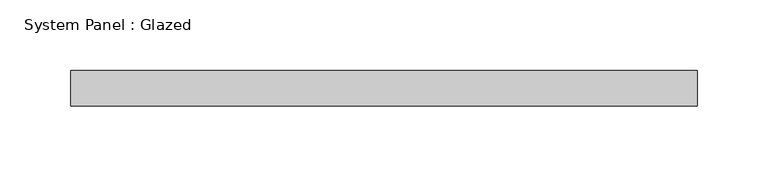
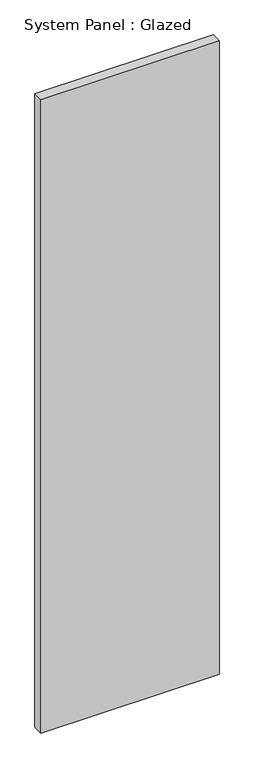
"""IFC4 building model written with IfcOpenShell, lengths in millimetres: plate geometry, System Panel : Glazed."""

from ifc_helpers import new_model, si_unit, origin, origin_with_axes, place, context, project, spatial, polyline, outline, extrude, source, transform, mapped, element, save


def system_panel_glazed_4ea5c58e(model_context):
    return source(origin(), model_context, "Body", "SweptSolid", [
        extrude(outline(polyline([(222.25, 19.05), (-222.25, 19.05), (-222.25, 44.45), (222.25, 44.45), (222.25, 19.05)])), origin_with_axes(), (0.0, 0.0, 1.0), 1669.4671151),
    ])


if __name__ == "__main__":
    model = new_model("IFC4")
    model_context = context("Model", 3, world=origin())
    ifc_project = project(units=[si_unit("LENGTHUNIT", "METRE", prefix="MILLI")], contexts=[model_context])
    site = spatial("IfcSite", under=ifc_project)
    building = spatial("IfcBuilding", under=site)
    placement = place(None, origin())
    system_panel_glazed_shape = system_panel_glazed_4ea5c58e(model_context)
    element("IfcPlate", 1, ObjectType="System Panel : Glazed", at=placement, inside=building, context=model_context, shape_type="MappedRepresentation", body=[
        mapped(system_panel_glazed_shape, transform((0.0, 0.0, 0.0), x_axis=(1.0, 0.0, 0.0), y_axis=(0.0, 1.0, 0.0), z_axis=(0.0, 0.0, 1.0))),
    ])
    save(model, "model.ifc")

# Revit data of these elements
# Type "System Panel : Glazed"
#   Construction Type Id = "GSP4R"
#   Analytic Construction = "1/8 in Pilkington single glazing"
#   Visual Light Transmittance = 0.9
#   Solar Heat Gain Coefficient = 0.86
#   Heat Transfer Coefficient (U) = 1.18115 BTU/(h·ft²·°F)
#   Define Thermal Properties by = 1
# Element 1 (IfcPlate, "System Panel : Glazed")
#   Materials on its faces: "Glass"
# Materials
#   "Glass": class "Glass", colour RGB 0 128 192, transparency 0.75, Description = "Soda Lime Glass", Cost = 0
